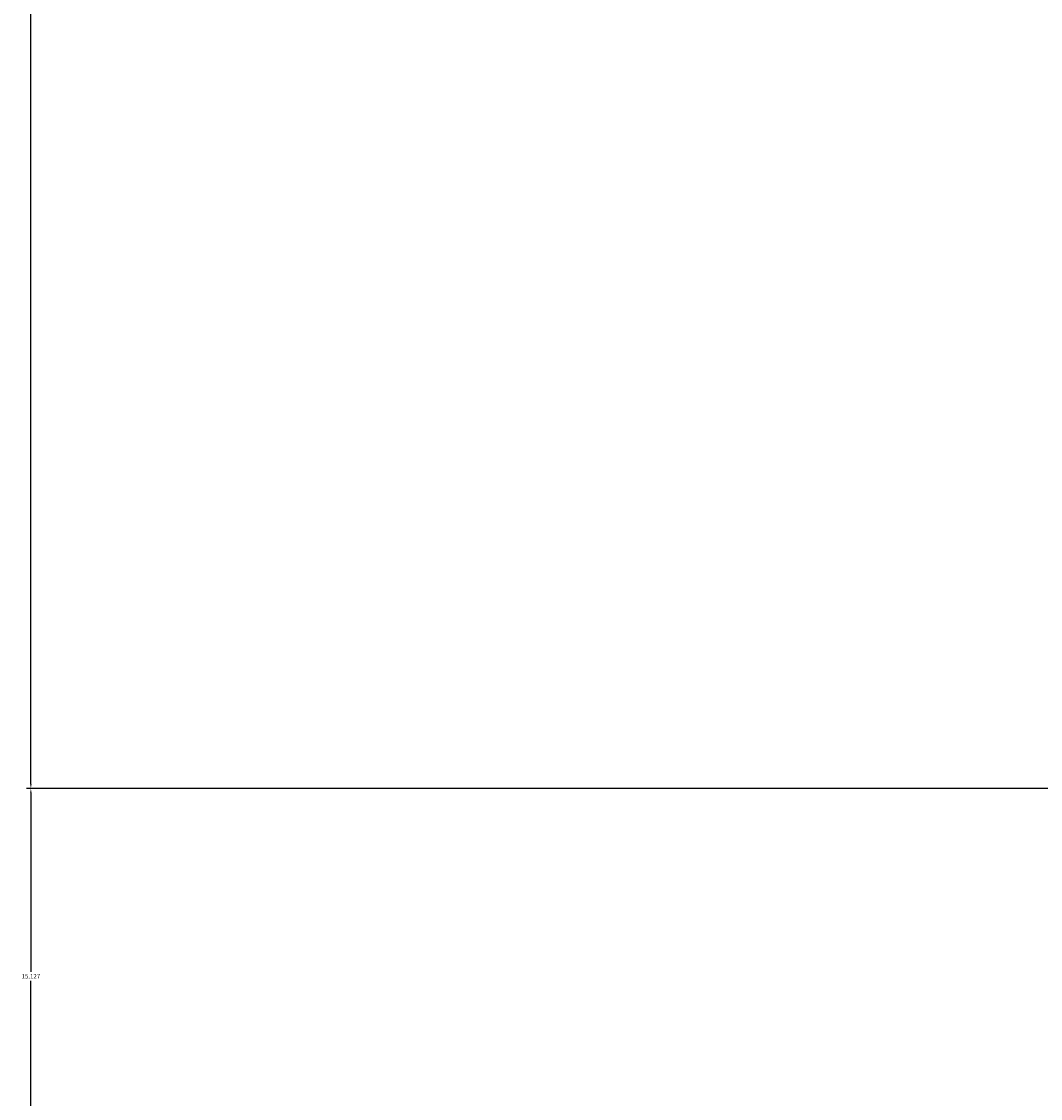
# Model space of a CAD drawing. Units: inches. Extents: x 738 to 1068, y 378 to 757.
# Tile 8 of 41: x 738 to 779, y 449 to 492. Entities that reach past the tile are written whole.
import ezdxf

# ---------------------------------------------------------------- set-up
doc = ezdxf.new("R2010")
doc.units = ezdxf.units.IN
doc.header["$MEASUREMENT"] = 0
doc.layers.add('A-ANNO-DIMS', color=2, linetype='Continuous', lineweight=18)
doc.styles.get("Standard").update_dxf_attribs({"font": 'arial.ttf'})
doc.dimstyles.get("Standard").update_dxf_attribs({"dimtxt": 0.18, "dimasz": 0.18, "dimexe": 0.18, "dimexo": 0.0625, "dimgap": 0.09, "dimtad": 0, "dimtih": 1, "dimtoh": 1, "dimdec": 4, "dimzin": 0, "dimdsep": 46, "dimtxsty": 'Standard', "dimcen": 0.09, "dimadec": 0, "dimazin": 0, "dimtfac": 1, "dimtdec": 4, "dimtofl": 0, "dimtmove": 0, "dimatfit": 3, "dimfxl": 1, "dimtolj": 1, "dimtzin": 0, "dimarcsym": 0})

# ---------------------------------------------------------------- blocks, each defined once
blk = doc.blocks.new('*D20')
at = {"layer": 'A-ANNO-DIMS', "color": 0, "lineweight": -2, "transparency": 16777216}
for p, q in [((781.427, 461.392), (738.194, 461.392)), ((738.374, 461.212), (738.374, 454.01)), ((738.374, 446.445), (738.374, 453.647)), ((781.422, 446.265), (738.194, 446.265))]:
    blk.add_line(p, q, dxfattribs=at)
at = {"layer": 'A-ANNO-DIMS', "color": 0, "transparency": 16777216}
for points in [[(738.344, 461.212), (738.404, 461.212), (738.374, 461.392)], [(738.344, 446.445), (738.404, 446.445), (738.374, 446.265)]]:
    blk.add_solid(points, dxfattribs=at)
at = {"layer": 'Defpoints', "color": 0, "transparency": 16777216}
for p in [(738.374, 461.392), (781.49, 461.392), (781.485, 446.265)]:
    blk.add_point(p, dxfattribs=at)
at = {"layer": 'A-ANNO-DIMS', "color": 0, "transparency": 16777216, "insert": (738.374, 453.829), "char_height": 0.18, "attachment_point": 5}
blk.add_mtext('\\A1;15.127', dxfattribs=at)
blk = doc.blocks.new('*D21')
at = {"layer": 'A-ANNO-DIMS', "color": 0, "lineweight": -2, "transparency": 16777216}
for p, q in [((781.427, 531.401), (738.194, 531.401)), ((738.374, 531.221), (738.374, 496.578)), ((738.374, 461.572), (738.374, 496.215)), ((781.427, 461.392), (738.194, 461.392))]:
    blk.add_line(p, q, dxfattribs=at)
at = {"layer": 'A-ANNO-DIMS', "color": 0, "transparency": 16777216}
for points in [[(738.344, 531.221), (738.404, 531.221), (738.374, 531.401)], [(738.344, 461.572), (738.404, 461.572), (738.374, 461.392)]]:
    blk.add_solid(points, dxfattribs=at)
at = {"layer": 'Defpoints', "color": 0, "transparency": 16777216}
for p in [(738.374, 531.401), (781.49, 531.401), (781.49, 461.392)]:
    blk.add_point(p, dxfattribs=at)
at = {"layer": 'A-ANNO-DIMS', "color": 0, "transparency": 16777216, "insert": (738.374, 496.396), "char_height": 0.18, "attachment_point": 5}
blk.add_mtext('\\A1;70.01', dxfattribs=at)

msp = doc.modelspace()

# ---------------------------------------------------------------- dimensions: what is measured, and where the dimension line sits
at = {"layer": 'A-ANNO-DIMS'}
for base, p1, p2, override, picture, middle in [((738.3736, 531.4009), (781.4897, 461.3919), (781.4897, 531.4009), {"dimdec": 2, "dimlfac": 1, "dimrnd": 0, "dimzin": 0, "dimdsep": 46, "dimlunit": 2}, '*D21', (738.3736, 496.3964)), ((738.3736, 461.3919), (781.4846, 446.2651), (781.4897, 461.3919), {"dimdec": 3, "dimlfac": 1, "dimrnd": 0, "dimzin": 0, "dimdsep": 46, "dimlunit": 2}, '*D20', (738.3736, 453.8285))]:
    dim = msp.add_linear_dim(base=base, p1=p1, p2=p2, angle=90, dimstyle='Standard', override=override, dxfattribs=at)
    dim.commit()
    dim.dimension.update_dxf_attribs({"geometry": picture, "text_midpoint": middle})

doc.saveas('drawing.dxf')
